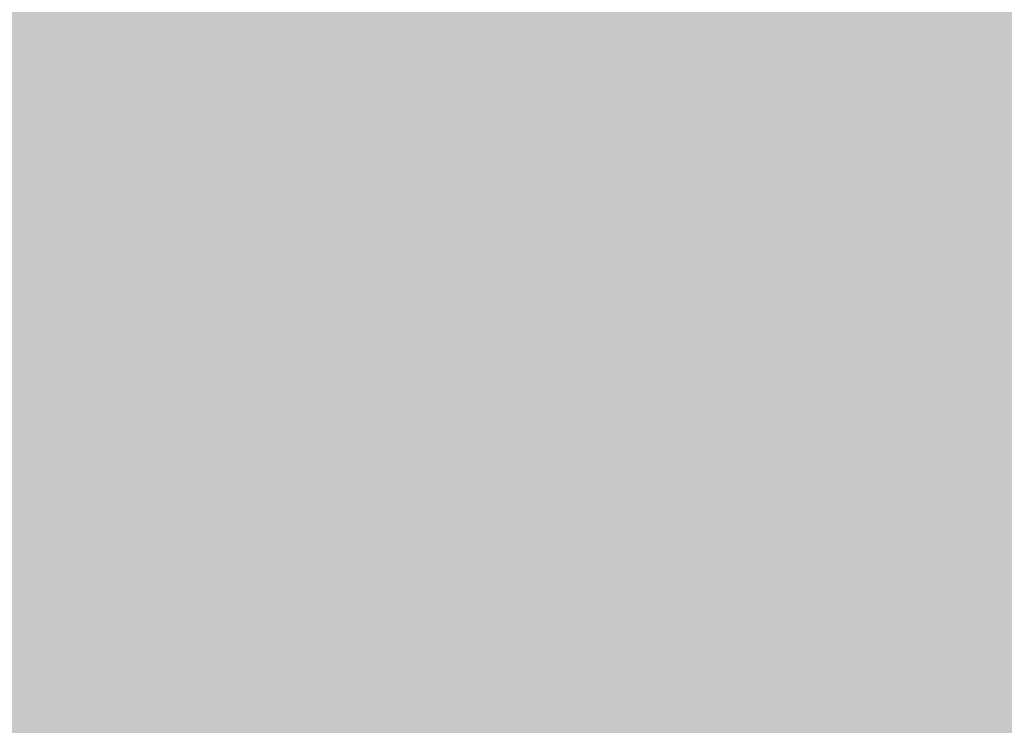
# Model space of a CAD drawing. Units: millimetres. Extents: x 0 to 2267, y 0 to 1823.
# Tile 77 of 256: x 1589.69 to 1600.37, y 1235.77 to 1243.41. Entities that reach past the tile are written whole.
import ezdxf

# ---------------------------------------------------------------- set-up
doc = ezdxf.new("R2010")
doc.units = ezdxf.units.MM
doc.header["$MEASUREMENT"] = 0
doc.layers.add('M-DIMS', color=2, linetype='Continuous', lineweight=25)
doc.layers.add('M-HATC', color=252, linetype='Continuous', lineweight=18)
doc.styles.get("Standard").update_dxf_attribs({"font": 'arial.ttf'})
doc.dimstyles.get("Standard").update_dxf_attribs({"dimtxt": 7, "dimasz": 4, "dimexe": 0.18, "dimexo": 0.0625, "dimgap": 0.09, "dimtad": 0, "dimdec": 0, "dimzin": 0, "dimdsep": 46, "dimtxsty": 'Standard', "dimcen": 0.09, "dimadec": 0, "dimazin": 0, "dimtfac": 1, "dimtdec": 0, "dimtofl": 0, "dimtmove": 0, "dimatfit": 3, "dimfxl": 1, "dimtolj": 1, "dimtzin": 0, "dimarcsym": 0})

# ---------------------------------------------------------------- blocks, each defined once
blk = doc.blocks.new('*D19')
at = {"layer": 'Defpoints', "color": 0, "transparency": 16777216}
for p in [(1605.34, 1483.304), (1445.529, 1333.885)]:
    blk.add_point(p, dxfattribs=at)
at = {"layer": 'M-DIMS', "color": 0, "lineweight": -2, "transparency": 16777216}
for p, q in [((1605.34, 1483.214), (1605.34, 1483.394)), ((1605.25, 1483.304), (1605.43, 1483.304)), ((1366.324, 1259.831), (1442.607, 1331.153))]:
    blk.add_line(p, q, dxfattribs=at)
at = {"layer": 'M-DIMS', "color": 0, "transparency": 16777216}
blk.add_solid([(1442.152, 1331.64), (1443.063, 1330.666), (1445.529, 1333.885)], dxfattribs=at)
at = {"layer": 'M-DIMS', "color": 0, "transparency": 16777216, "insert": (1349.643, 1244.233), "char_height": 7, "attachment_point": 5, "rotation": 43.0753}
blk.add_mtext('\\A1;2X R218.8', dxfattribs=at)

msp = doc.modelspace()

# ---------------------------------------------------------------- hatches: boundary and pattern name
at = {"layer": 'M-HATC'}
h = msp.add_hatch(color=256, dxfattribs=at)
h.dxf.hatch_style = 1
h.paths.add_polyline_path([(2065.771, 1618.062, 0.236068), (2055.771, 1638.062), (1381.087, 1638.062, 0.236068), (1371.087, 1618.062), (1371.087, 1603.062), (2055.771, 1603.062), (2065.771, 1603.062)])
h.paths.add_polyline_path([(2062.772, 1550.296), (2062.772, 1560.296), (1374.086, 1560.296), (1374.086, 1550.296), (1374.086, 1540.296), (1384.086, 1540.296), (1389.086, 1540.296), (2062.772, 1540.296)])
h.paths.add_polyline_path([(1930.929, 1282.766), (1505.929, 1282.766), (1587.628, 1235.597, 0.131652), (1600.128, 1232.247), (1836.73, 1232.247, 0.131652), (1849.23, 1235.597)])
h.paths.add_polyline_path([(1930.929, 1117.417), (1905.929, 1117.417), (1505.929, 1117.417), (1505.929, 1077.417), (1930.929, 1077.417)])
h = msp.add_hatch(color=256, dxfattribs=at)
h.dxf.hatch_style = 1
h.paths.add_polyline_path([(2055.771, 1603.062), (1381.087, 1603.062), (1381.087, 1598.062), (2055.771, 1598.062)])
h.paths.add_polyline_path([(2055.771, 1598.062), (1381.087, 1598.062), (1381.087, 1593.062), (2055.771, 1593.062)])
h.paths.add_polyline_path([(2051.307, 1536.761), (1385.55, 1536.761), (1385.55, 1526.761), (1387.55, 1526.761), (1388.537, 1525.053), (1385.332, 1521.233), (1385.332, 1521.223), (2050.254, 1522.749), (2048.321, 1525.053), (2049.307, 1526.761), (2051.307, 1526.761)])
edge = h.paths.add_edge_path()
edge.add_arc((1847.535, 1379.149), 135, 222.60306, 222.89085, ccw=False)
edge.add_line((1748.166, 1287.766), (1683.092, 1287.766))
edge.add_arc((1583.724, 1379.149), 135, 317.10915, 317.39694, ccw=False)
edge.add_arc((1678.969, 1290.671), 5, 222.8909, 317.1091, ccw=False)
edge.add_arc((1774.213, 1379.149), 135, 222.60306, 222.89085, ccw=False)
edge.add_line((1674.845, 1287.766), (1609.771, 1287.766))
edge.add_arc((1510.403, 1379.149), 135, 317.10915, 317.39694, ccw=False)
edge.add_arc((1605.647, 1290.671), 5, 222.8909, 317.1091, ccw=False)
edge.add_arc((1700.892, 1379.149), 135, 222.60306, 222.89085, ccw=False)
edge.add_line((1601.524, 1287.766), (1536.45, 1287.766))
edge.add_arc((1437.081, 1379.149), 135, 317.10915, 317.39694, ccw=False)
edge.add_arc((1532.326, 1290.671), 5, 222.8909, 317.1091, ccw=False)
edge.add_arc((1627.571, 1379.149), 135, 222.60306, 222.89085, ccw=False)
edge.add_line((1528.203, 1287.766), (1505.929, 1287.766))
edge.add_spline(control_points=[(1505.929, 1287.766), (1504.262, 1287.766), (1504.262, 1282.766), (1505.929, 1282.766)], knot_values=[0, 0, 0, 0, 5, 5, 5, 5], degree=3, periodic=0)
edge.add_line((1505.929, 1282.766), (1930.929, 1282.766))
edge.add_spline(control_points=[(1930.929, 1282.766), (1932.596, 1282.766), (1932.596, 1287.766), (1930.929, 1287.766)], knot_values=[0, 0, 0, 0, 5, 5, 5, 5], degree=3, periodic=0)
edge.add_line((1930.929, 1287.766), (1903.056, 1287.766))
edge.add_arc((1803.688, 1379.149), 135, 317.10915, 317.39694, ccw=False)
edge.add_arc((1898.932, 1290.671), 5, 222.8909, 317.1091, ccw=False)
edge.add_arc((1994.177, 1379.149), 135, 222.60306, 222.89085, ccw=False)
edge.add_line((1894.809, 1287.766), (1829.735, 1287.766))
edge.add_arc((1730.366, 1379.149), 135, 317.10915, 317.39694, ccw=False)
edge.add_arc((1825.611, 1290.671), 5, 222.8909, 317.1091, ccw=False)
edge.add_arc((1920.856, 1379.149), 135, 222.60306, 222.89085, ccw=False)
edge.add_line((1821.487, 1287.766), (1756.413, 1287.766))
edge.add_arc((1657.045, 1379.149), 135, 317.10915, 317.39694, ccw=False)
edge.add_arc((1752.29, 1290.671), 5, 222.8909, 317.1091, ccw=False)
edge = h.paths.add_edge_path()
edge.add_spline(control_points=[(1843.429, 1227.247), (1845.096, 1227.247), (1845.096, 1232.247), (1843.429, 1232.247)], knot_values=[0, 0, 0, 0, 5, 5, 5, 5], degree=3, periodic=0)
edge.add_line((1843.429, 1232.247), (1593.429, 1232.247))
edge.add_spline(control_points=[(1593.429, 1232.247), (1591.762, 1232.247), (1591.762, 1227.247), (1593.429, 1227.247)], knot_values=[0, 0, 0, 0, 5, 5, 5, 5], degree=3, periodic=0)
edge.add_line((1593.429, 1227.247), (1843.429, 1227.247))
h.paths.add_polyline_path([(1905.929, 1127.417), (1530.929, 1127.417, 0.414214), (1520.929, 1117.417), (1530.929, 1117.417), (1915.929, 1117.417, 0.414214)])
edge = h.paths.add_edge_path()
edge.add_arc((1397.086, 1498.408), 12.73, 90.7821, 190.8787, ccw=False)
edge.add_line((1396.912, 1511.136), (1428.01, 1511.349))
edge.add_line((1428.01, 1511.349), (1433.01, 1511.349))
edge.add_line((1433.01, 1511.349), (1434.439, 1511.349))
edge.add_arc((1419.474, 1498.08), 20, 41.561, 74.0821)
edge.add_line((1424.959, 1517.314), (1399.935, 1517.256))
edge.add_spline(control_points=[(1399.931, 1517.256), (1399.884, 1517.213), (1399.833, 1517.169), (1399.777, 1517.124)], knot_values=[11.567499, 11.567499, 11.567499, 11.567499, 11.814249, 11.814249, 11.814249, 11.814249], degree=3, periodic=0)
edge.add_spline(control_points=[(1399.633, 1517.01), (1399.583, 1516.972), (1399.531, 1516.934), (1399.476, 1516.895)], knot_values=[11.167718, 11.167718, 11.167718, 11.167718, 11.365188, 11.365188, 11.365188, 11.365188], degree=3, periodic=0)
edge.add_spline(control_points=[(1399.34, 1516.8), (1399.151, 1516.672), (1398.938, 1516.538), (1398.704, 1516.399)], knot_values=[10.376405, 10.376405, 10.376405, 10.376405, 11.00994, 11.00994, 11.00994, 11.00994], degree=3, periodic=0)
edge.add_spline(control_points=[(1398.657, 1516.372), (1398.579, 1516.326), (1398.498, 1516.28), (1398.415, 1516.233)], knot_values=[10.125175, 10.125175, 10.125175, 10.125175, 10.334406, 10.334406, 10.334406, 10.334406], degree=3, periodic=0)
edge.add_spline(control_points=[(1398.264, 1516.149), (1398.196, 1516.111), (1398.126, 1516.073), (1398.055, 1516.035)], knot_values=[9.832246, 9.832246, 9.832246, 9.832246, 9.999658, 9.999658, 9.999658, 9.999658], degree=3, periodic=0)
edge.add_spline(control_points=[(1397.999, 1516.005), (1397.731, 1515.862), (1397.446, 1515.717), (1397.147, 1515.571)], knot_values=[9.161808, 9.161808, 9.161808, 9.161808, 9.787769, 9.787769, 9.787769, 9.787769], degree=3, periodic=0)
edge.add_spline(control_points=[(1397.147, 1515.571), (1396.842, 1515.423), (1396.522, 1515.274), (1396.191, 1515.126)], knot_values=[8.524455, 8.524455, 8.524455, 8.524455, 9.161808, 9.161808, 9.161808, 9.161808], degree=3, periodic=0)
edge.add_spline(control_points=[(1396.078, 1515.076), (1395.985, 1515.035), (1395.892, 1514.994), (1395.798, 1514.953)], knot_values=[8.275193, 8.275193, 8.275193, 8.275193, 8.451726, 8.451726, 8.451726, 8.451726], degree=3, periodic=0)
edge.add_spline(control_points=[(1395.602, 1514.869), (1395.5, 1514.826), (1395.397, 1514.782), (1395.293, 1514.739)], knot_values=[7.962917, 7.962917, 7.962917, 7.962917, 8.152764, 8.152764, 8.152764, 8.152764], degree=3, periodic=0)
edge.add_spline(control_points=[(1395.212, 1514.706), (1394.828, 1514.547), (1394.435, 1514.393), (1394.036, 1514.244)], knot_values=[7.21254, 7.21254, 7.21254, 7.21254, 7.913148, 7.913148, 7.913148, 7.913148], degree=3, periodic=0)
edge.add_spline(control_points=[(1394.036, 1514.244), (1393.708, 1514.121), (1393.375, 1514.003), (1393.043, 1513.889)], knot_values=[6.633733, 6.633733, 6.633733, 6.633733, 7.21254, 7.21254, 7.21254, 7.21254], degree=3, periodic=0)
edge.add_spline(control_points=[(1392.821, 1513.815), (1392.72, 1513.781), (1392.618, 1513.748), (1392.517, 1513.715)], knot_values=[6.328796, 6.328796, 6.328796, 6.328796, 6.505493, 6.505493, 6.505493, 6.505493], degree=3, periodic=0)
edge.add_spline(control_points=[(1392.517, 1513.715), (1392.319, 1513.652), (1392.121, 1513.59), (1391.924, 1513.531)], knot_values=[5.984605, 5.984605, 5.984605, 5.984605, 6.328796, 6.328796, 6.328796, 6.328796], degree=3, periodic=0)
edge.add_spline(control_points=[(1391.792, 1513.491), (1391.312, 1513.35), (1390.838, 1513.224), (1390.378, 1513.117)], knot_values=[5.066697, 5.066697, 5.066697, 5.066697, 5.907055, 5.907055, 5.907055, 5.907055], degree=3, periodic=0)
edge.add_spline(control_points=[(1390.378, 1513.117), (1390.18, 1513.071), (1389.984, 1513.028), (1389.791, 1512.99)], knot_values=[4.70367, 4.70367, 4.70367, 4.70367, 5.066695, 5.066695, 5.066695, 5.066695], degree=3, periodic=0)
edge.add_spline(control_points=[(1389.422, 1512.92), (1389.246, 1512.889), (1389.073, 1512.862), (1388.904, 1512.838)], knot_values=[4.130571, 4.130571, 4.130571, 4.130571, 4.469816, 4.469816, 4.469816, 4.469816], degree=3, periodic=0)
edge.add_spline(control_points=[(1388.904, 1512.838), (1388.591, 1512.795), (1388.291, 1512.764), (1388.007, 1512.749)], knot_values=[3.504031, 3.504031, 3.504031, 3.504031, 4.130571, 4.130571, 4.130571, 4.130571], degree=3, periodic=0)
edge.add_spline(control_points=[(1387.936, 1512.746), (1387.854, 1512.742), (1387.773, 1512.74), (1387.694, 1512.739)], knot_values=[3.268866, 3.268866, 3.268866, 3.268866, 3.451164, 3.451164, 3.451164, 3.451164], degree=3, periodic=0)
edge.add_spline(control_points=[(1387.335, 1512.744), (1387.208, 1512.75), (1387.085, 1512.76), (1386.967, 1512.774)], knot_values=[2.670686, 2.670686, 2.670686, 2.670686, 2.984, 2.984, 2.984, 2.984], degree=3, periodic=0)
edge.add_spline(control_points=[(1386.833, 1512.792), (1386.821, 1512.794), (1386.809, 1512.796), (1386.797, 1512.798)], knot_values=[2.516981, 2.516981, 2.516981, 2.516981, 2.549528, 2.549528, 2.549528, 2.549528], degree=3, periodic=0)
edge.add_spline(control_points=[(1386.453, 1512.873), (1386.426, 1512.881), (1386.399, 1512.889), (1386.373, 1512.897)], knot_values=[2.095869, 2.095869, 2.095869, 2.095869, 2.17941, 2.17941, 2.17941, 2.17941], degree=3, periodic=0)
edge.add_spline(control_points=[(1386.069, 1513.019), (1386.063, 1513.022), (1386.058, 1513.025), (1386.052, 1513.028)], knot_values=[1.72453, 1.72453, 1.72453, 1.72453, 1.745933, 1.745933, 1.745933, 1.745933], degree=3, periodic=0)
edge.add_arc((1399.474, 1498.08), 20, 131.8243, 180)
edge.add_arc((1630.334, 1505.548), 250.971, 181.70518, 236.42798)
edge.add_arc((1605.34, 1483.304), 218.782, 238.66083, 243.34961)
edge.add_arc((1647.091, 1510.359), 262.899, 183.12984, 237.85344, ccw=False)
h.paths.add_polyline_path([(1406.537, 1391.964, 0.149382), (1491.551, 1296.442, -0.129517)], flags=17)
edge = h.paths.add_edge_path()
edge.add_arc((2037.384, 1498.08), 20, 0, 48.2659)
edge.add_spline(control_points=[(2050.697, 1513.005), (2050.651, 1512.985), (2050.603, 1512.966), (2050.554, 1512.948)], knot_values=[1.835652, 1.835652, 1.835652, 1.835652, 2.000781, 2.000781, 2.000781, 2.000781], degree=3, periodic=0)
edge.add_spline(control_points=[(2050.462, 1512.917), (2050.479, 1512.922), (2050.496, 1512.928), (2050.513, 1512.934)], knot_values=[2.045477, 2.045477, 2.045477, 2.045477, 2.101389, 2.101389, 2.101389, 2.101389], degree=3, periodic=0)
edge.add_spline(control_points=[(2050.129, 1512.834), (2050.198, 1512.847), (2050.266, 1512.862), (2050.331, 1512.879)], knot_values=[2.237629, 2.237629, 2.237629, 2.237629, 2.435841, 2.435841, 2.435841, 2.435841], degree=3, periodic=0)
edge.add_spline(control_points=[(2050.095, 1512.828), (2050.106, 1512.83), (2050.118, 1512.832), (2050.129, 1512.834)], knot_values=[2.435841, 2.435841, 2.435841, 2.435841, 2.468321, 2.468321, 2.468321, 2.468321], degree=3, periodic=0)
edge.add_spline(control_points=[(2049.784, 1512.785), (2049.855, 1512.792), (2049.924, 1512.801), (2049.992, 1512.811)], knot_values=[2.563852, 2.563852, 2.563852, 2.563852, 2.748541, 2.748541, 2.748541, 2.748541], degree=3, periodic=0)
edge.add_spline(control_points=[(2049.405, 1512.762), (2049.536, 1512.765), (2049.663, 1512.773), (2049.784, 1512.785)], knot_values=[2.748541, 2.748541, 2.748541, 2.748541, 3.064882, 3.064882, 3.064882, 3.064882], degree=3, periodic=0)
edge.add_spline(control_points=[(2049.17, 1512.76), (2049.234, 1512.759), (2049.297, 1512.759), (2049.358, 1512.761)], knot_values=[3.102309, 3.102309, 3.102309, 3.102309, 3.2503, 3.2503, 3.2503, 3.2503], degree=3, periodic=0)
edge.add_spline(control_points=[(2048.857, 1512.769), (2048.964, 1512.764), (2049.068, 1512.761), (2049.17, 1512.76)], knot_values=[3.2503, 3.2503, 3.2503, 3.2503, 3.486069, 3.486069, 3.486069, 3.486069], degree=3, periodic=0)
edge.add_spline(control_points=[(2048.692, 1512.779), (2048.373, 1512.801), (2048.035, 1512.841), (2047.682, 1512.897)], knot_values=[3.606429, 3.606429, 3.606429, 3.606429, 4.2989, 4.2989, 4.2989, 4.2989], degree=3, periodic=0)
edge.add_spline(control_points=[(2047.682, 1512.897), (2047.546, 1512.919), (2047.408, 1512.942), (2047.268, 1512.969)], knot_values=[4.2989, 4.2989, 4.2989, 4.2989, 4.565769, 4.565769, 4.565769, 4.565769], degree=3, periodic=0)
edge.add_spline(control_points=[(2047.268, 1512.969), (2047.145, 1512.991), (2047.021, 1513.016), (2046.895, 1513.042)], knot_values=[4.565769, 4.565769, 4.565769, 4.565769, 4.799971, 4.799971, 4.799971, 4.799971], degree=3, periodic=0)
edge.add_spline(control_points=[(2046.895, 1513.042), (2046.529, 1513.119), (2046.151, 1513.209), (2045.768, 1513.311)], knot_values=[4.799971, 4.799971, 4.799971, 4.799971, 5.483718, 5.483718, 5.483718, 5.483718], degree=3, periodic=0)
edge.add_spline(control_points=[(2045.768, 1513.311), (2045.372, 1513.415), (2044.97, 1513.532), (2044.566, 1513.659)], knot_values=[5.483718, 5.483718, 5.483718, 5.483718, 6.187866, 6.187866, 6.187866, 6.187866], degree=3, periodic=0)
edge.add_spline(control_points=[(2044.566, 1513.659), (2044.415, 1513.706), (2044.263, 1513.755), (2044.112, 1513.805)], knot_values=[6.187866, 6.187866, 6.187866, 6.187866, 6.451551, 6.451551, 6.451551, 6.451551], degree=3, periodic=0)
edge.add_spline(control_points=[(2044.112, 1513.805), (2043.997, 1513.843), (2043.882, 1513.881), (2043.767, 1513.92)], knot_values=[6.451551, 6.451551, 6.451551, 6.451551, 6.651434, 6.651434, 6.651434, 6.651434], degree=3, periodic=0)
edge.add_spline(control_points=[(2043.767, 1513.92), (2043.372, 1514.055), (2042.977, 1514.198), (2042.589, 1514.346)], knot_values=[6.651434, 6.651434, 6.651434, 6.651434, 7.338879, 7.338879, 7.338879, 7.338879], degree=3, periodic=0)
edge.add_spline(control_points=[(2042.589, 1514.346), (2042.164, 1514.507), (2041.746, 1514.675), (2041.341, 1514.846)], knot_values=[7.338879, 7.338879, 7.338879, 7.338879, 8.089209, 8.089209, 8.089209, 8.089209], degree=3, periodic=0)
edge.add_spline(control_points=[(2041.341, 1514.846), (2041.103, 1514.946), (2040.869, 1515.048), (2040.64, 1515.15)], knot_values=[8.089209, 8.089209, 8.089209, 8.089209, 8.529587, 8.529587, 8.529587, 8.529587], degree=3, periodic=0)
edge.add_spline(control_points=[(2040.51, 1515.209), (2040.082, 1515.402), (2039.675, 1515.597), (2039.295, 1515.789)], knot_values=[8.613818, 8.613818, 8.613818, 8.613818, 9.44571, 9.44571, 9.44571, 9.44571], degree=3, periodic=0)
edge.add_spline(control_points=[(2039.295, 1515.789), (2039.062, 1515.907), (2038.839, 1516.025), (2038.629, 1516.14)], knot_values=[9.44571, 9.44571, 9.44571, 9.44571, 9.956404, 9.956404, 9.956404, 9.956404], degree=3, periodic=0)
edge.add_spline(control_points=[(2038.629, 1516.14), (2038.519, 1516.2), (2038.412, 1516.26), (2038.309, 1516.319)], knot_values=[9.956404, 9.956404, 9.956404, 9.956404, 10.223542, 10.223542, 10.223542, 10.223542], degree=3, periodic=0)
edge.add_spline(control_points=[(2038.309, 1516.319), (2038.214, 1516.374), (2038.122, 1516.428), (2038.033, 1516.481)], knot_values=[10.223542, 10.223542, 10.223542, 10.223542, 10.47051, 10.47051, 10.47051, 10.47051], degree=3, periodic=0)
edge.add_spline(control_points=[(2038.033, 1516.481), (2037.786, 1516.63), (2037.564, 1516.773), (2037.372, 1516.909)], knot_values=[10.47051, 10.47051, 10.47051, 10.47051, 11.15767, 11.15767, 11.15767, 11.15767], degree=3, periodic=0)
edge.add_spline(control_points=[(2037.372, 1516.909), (2037.279, 1516.975), (2037.193, 1517.04), (2037.114, 1517.102)], knot_values=[11.15767, 11.15767, 11.15767, 11.15767, 11.49227, 11.49227, 11.49227, 11.49227], degree=3, periodic=0)
edge.add_spline(control_points=[(2036.856, 1517.326), (2036.915, 1517.269), (2036.981, 1517.21), (2037.056, 1517.149)], knot_values=[11.577341, 11.577341, 11.577341, 11.577341, 11.91035, 11.91035, 11.91035, 11.91035], degree=3, periodic=0)
edge.add_spline(control_points=[(2036.807, 1517.375), (2036.823, 1517.359), (2036.839, 1517.342), (2036.856, 1517.326)], knot_values=[11.91035, 11.91035, 11.91035, 11.91035, 12.007402, 12.007402, 12.007402, 12.007402], degree=3, periodic=0)
edge.add_spline(control_points=[(2036.702, 1517.494), (2036.71, 1517.483), (2036.72, 1517.472), (2036.729, 1517.461)], knot_values=[12.184155, 12.184155, 12.184155, 12.184155, 12.255409, 12.255409, 12.255409, 12.255409], degree=3, periodic=0)
edge.add_spline(control_points=[(2036.616, 1517.621), (2036.62, 1517.613), (2036.624, 1517.606), (2036.629, 1517.598)], knot_values=[12.487913, 12.487913, 12.487913, 12.487913, 12.541035, 12.541035, 12.541035, 12.541035], degree=3, periodic=0)
edge.add_spline(control_points=[(2036.563, 1517.786), (2036.564, 1517.779), (2036.564, 1517.773), (2036.565, 1517.766)], knot_values=[12.911761, 12.911761, 12.911761, 12.911761, 12.968286, 12.968286, 12.968286, 12.968286], degree=3, periodic=0)
edge.add_spline(control_points=[(2036.617, 1517.93), (2036.612, 1517.926), (2036.609, 1517.921), (2036.605, 1517.916)], knot_values=[13.382527, 13.382527, 13.382527, 13.382527, 13.433791, 13.433791, 13.433791, 13.433791], degree=3, periodic=0)
edge.add_spline(control_points=[(2036.749, 1518.017), (2036.736, 1518.012), (2036.724, 1518.006), (2036.712, 1518)], knot_values=[13.726299, 13.726299, 13.726299, 13.726299, 13.809928, 13.809928, 13.809928, 13.809928], degree=3, periodic=0)
edge.add_spline(control_points=[(2036.86, 1518.053), (2036.839, 1518.047), (2036.818, 1518.042), (2036.799, 1518.035)], knot_values=[13.910887, 13.910887, 13.910887, 13.910887, 14.02153, 14.02153, 14.02153, 14.02153], degree=3, periodic=0)
edge.add_line((2036.964, 1518.08), (2032.384, 1518.08))
edge.add_line((2032.384, 1518.08), (2027.384, 1518.08))
edge.add_line((2027.384, 1518.08), (2022.384, 1518.08))
edge.add_line((2022.384, 1518.08), (2017.384, 1518.08))
edge.add_arc((2017.384, 1498.08), 20, 90, 138.439)
edge.add_line((2002.419, 1511.349), (2003.848, 1511.349))
edge.add_line((2003.848, 1511.349), (2008.848, 1511.349))
edge.add_line((2008.848, 1511.349), (2039.772, 1511.138))
edge.add_arc((2039.772, 1498.408), 12.73, -10.8787, 90, ccw=False)
edge.add_arc((1789.767, 1510.359), 262.899, 302.14656, 356.87016, ccw=False)
edge.add_arc((1831.518, 1483.304), 218.782, 296.65039, 301.33917)
edge.add_arc((1806.524, 1505.548), 250.971, 303.57202, 358.29482)
h.paths.add_polyline_path([(2030.321, 1391.964, -0.129517), (1945.307, 1296.442, 0.149382)], flags=17)
edge = h.paths.add_edge_path()
edge.add_spline(control_points=[(2037.246, 1518.082), (2037.29, 1518.081), (2037.336, 1518.08), (2037.384, 1518.08)], knot_values=[0.000012, 0.000012, 0.000012, 0.000012, 0.144754, 0.144754, 0.144754, 0.144754], degree=3, periodic=0)
edge.add_line((2037.336, 1518.08), (2037.01, 1518.08))
edge.add_spline(control_points=[(2037.01, 1518.08), (2036.982, 1518.077), (2036.956, 1518.073), (2036.931, 1518.068)], knot_values=[14.13465, 14.13465, 14.13465, 14.13465, 14.247197, 14.247197, 14.247197, 14.247197], degree=3, periodic=0)
edge.add_spline(control_points=[(2036.931, 1518.068), (2036.928, 1518.067), (2036.924, 1518.067), (2036.921, 1518.066)], knot_values=[14.118315, 14.118315, 14.118315, 14.118315, 14.13465, 14.13465, 14.13465, 14.13465], degree=3, periodic=0)
edge.add_spline(control_points=[(2036.921, 1518.066), (2036.912, 1518.064), (2036.903, 1518.063), (2036.895, 1518.061)], knot_values=[14.078086, 14.078086, 14.078086, 14.078086, 14.118315, 14.118315, 14.118315, 14.118315], degree=3, periodic=0)
edge.add_spline(control_points=[(2036.895, 1518.061), (2036.883, 1518.058), (2036.872, 1518.056), (2036.86, 1518.053)], knot_values=[14.02153, 14.02153, 14.02153, 14.02153, 14.078086, 14.078086, 14.078086, 14.078086], degree=3, periodic=0)
edge.add_spline(control_points=[(2036.86, 1518.053), (2036.839, 1518.047), (2036.818, 1518.042), (2036.799, 1518.035)], knot_values=[13.910887, 13.910887, 13.910887, 13.910887, 14.02153, 14.02153, 14.02153, 14.02153], degree=3, periodic=0)
edge.add_spline(control_points=[(2036.799, 1518.035), (2036.798, 1518.035), (2036.797, 1518.035), (2036.797, 1518.035)], knot_values=[13.906906, 13.906906, 13.906906, 13.906906, 13.910887, 13.910887, 13.910887, 13.910887], degree=3, periodic=0)
edge.add_spline(control_points=[(2036.797, 1518.035), (2036.788, 1518.032), (2036.78, 1518.029), (2036.772, 1518.026)], knot_values=[13.857826, 13.857826, 13.857826, 13.857826, 13.906906, 13.906906, 13.906906, 13.906906], degree=3, periodic=0)
edge.add_spline(control_points=[(2036.772, 1518.026), (2036.764, 1518.023), (2036.756, 1518.02), (2036.749, 1518.017)], knot_values=[13.809928, 13.809928, 13.809928, 13.809928, 13.857826, 13.857826, 13.857826, 13.857826], degree=3, periodic=0)
edge.add_spline(control_points=[(2036.749, 1518.017), (2036.736, 1518.012), (2036.724, 1518.006), (2036.712, 1518)], knot_values=[13.726299, 13.726299, 13.726299, 13.726299, 13.809928, 13.809928, 13.809928, 13.809928], degree=3, periodic=0)
edge.add_spline(control_points=[(2036.712, 1518), (2036.712, 1518), (2036.712, 1518), (2036.711, 1518)], knot_values=[13.723993, 13.723993, 13.723993, 13.723993, 13.726299, 13.726299, 13.726299, 13.726299], degree=3, periodic=0)
edge.add_spline(control_points=[(2036.711, 1518), (2036.706, 1517.997), (2036.701, 1517.994), (2036.696, 1517.992)], knot_values=[13.686536, 13.686536, 13.686536, 13.686536, 13.723993, 13.723993, 13.723993, 13.723993], degree=3, periodic=0)
edge.add_spline(control_points=[(2036.696, 1517.992), (2036.692, 1517.989), (2036.687, 1517.987), (2036.683, 1517.984)], knot_values=[13.651251, 13.651251, 13.651251, 13.651251, 13.686536, 13.686536, 13.686536, 13.686536], degree=3, periodic=0)
edge.add_spline(control_points=[(2036.683, 1517.984), (2036.676, 1517.98), (2036.67, 1517.976), (2036.664, 1517.971)], knot_values=[13.596804, 13.596804, 13.596804, 13.596804, 13.651251, 13.651251, 13.651251, 13.651251], degree=3, periodic=0)
edge.add_spline(control_points=[(2036.664, 1517.971), (2036.664, 1517.971), (2036.663, 1517.971), (2036.663, 1517.971)], knot_values=[13.593956, 13.593956, 13.593956, 13.593956, 13.596804, 13.596804, 13.596804, 13.596804], degree=3, periodic=0)
edge.add_spline(control_points=[(2036.663, 1517.971), (2036.66, 1517.969), (2036.658, 1517.967), (2036.655, 1517.965)], knot_values=[13.570322, 13.570322, 13.570322, 13.570322, 13.593956, 13.593956, 13.593956, 13.593956], degree=3, periodic=0)
edge.add_spline(control_points=[(2036.655, 1517.965), (2036.653, 1517.963), (2036.65, 1517.961), (2036.647, 1517.959)], knot_values=[13.545477, 13.545477, 13.545477, 13.545477, 13.570322, 13.570322, 13.570322, 13.570322], degree=3, periodic=0)
edge.add_spline(control_points=[(2036.647, 1517.959), (2036.647, 1517.959), (2036.647, 1517.959), (2036.647, 1517.959)], knot_values=[13.543931, 13.543931, 13.543931, 13.543931, 13.545477, 13.545477, 13.545477, 13.545477], degree=3, periodic=0)
edge.add_spline(control_points=[(2036.647, 1517.959), (2036.641, 1517.954), (2036.636, 1517.949), (2036.631, 1517.945)], knot_values=[13.488237, 13.488237, 13.488237, 13.488237, 13.543931, 13.543931, 13.543931, 13.543931], degree=3, periodic=0)
edge.add_spline(control_points=[(2036.631, 1517.945), (2036.628, 1517.942), (2036.626, 1517.94), (2036.623, 1517.937)], knot_values=[13.460307, 13.460307, 13.460307, 13.460307, 13.488237, 13.488237, 13.488237, 13.488237], degree=3, periodic=0)
edge.add_spline(control_points=[(2036.623, 1517.937), (2036.622, 1517.936), (2036.62, 1517.934), (2036.618, 1517.932)], knot_values=[13.439712, 13.439712, 13.439712, 13.439712, 13.460307, 13.460307, 13.460307, 13.460307], degree=3, periodic=0)
edge.add_spline(control_points=[(2036.618, 1517.932), (2036.618, 1517.931), (2036.617, 1517.931), (2036.617, 1517.93)], knot_values=[13.433791, 13.433791, 13.433791, 13.433791, 13.439712, 13.439712, 13.439712, 13.439712], degree=3, periodic=0)
edge.add_spline(control_points=[(2036.617, 1517.93), (2036.612, 1517.926), (2036.609, 1517.921), (2036.605, 1517.916)], knot_values=[13.382527, 13.382527, 13.382527, 13.382527, 13.433791, 13.433791, 13.433791, 13.433791], degree=3, periodic=0)
edge.add_spline(control_points=[(2036.605, 1517.916), (2036.603, 1517.913), (2036.6, 1517.91), (2036.598, 1517.907)], knot_values=[13.350017, 13.350017, 13.350017, 13.350017, 13.382527, 13.382527, 13.382527, 13.382527], degree=3, periodic=0)
edge.add_spline(control_points=[(2036.598, 1517.907), (2036.597, 1517.906), (2036.596, 1517.904), (2036.595, 1517.903)], knot_values=[13.333922, 13.333922, 13.333922, 13.333922, 13.350017, 13.350017, 13.350017, 13.350017], degree=3, periodic=0)
edge.add_spline(control_points=[(2036.595, 1517.903), (2036.595, 1517.902), (2036.594, 1517.901), (2036.593, 1517.9)], knot_values=[13.323828, 13.323828, 13.323828, 13.323828, 13.333922, 13.333922, 13.333922, 13.333922], degree=3, periodic=0)
edge.add_spline(control_points=[(2036.593, 1517.9), (2036.59, 1517.895), (2036.588, 1517.891), (2036.585, 1517.886)], knot_values=[13.277545, 13.277545, 13.277545, 13.277545, 13.323828, 13.323828, 13.323828, 13.323828], degree=3, periodic=0)
edge.add_spline(control_points=[(2036.585, 1517.886), (2036.584, 1517.883), (2036.582, 1517.879), (2036.58, 1517.875)], knot_values=[13.240119, 13.240119, 13.240119, 13.240119, 13.277545, 13.277545, 13.277545, 13.277545], degree=3, periodic=0)
edge.add_spline(control_points=[(2036.58, 1517.875), (2036.58, 1517.874), (2036.579, 1517.873), (2036.578, 1517.872)], knot_values=[13.228211, 13.228211, 13.228211, 13.228211, 13.240119, 13.240119, 13.240119, 13.240119], degree=3, periodic=0)
edge.add_spline(control_points=[(2036.578, 1517.872), (2036.578, 1517.87), (2036.577, 1517.869), (2036.577, 1517.868)], knot_values=[13.215717, 13.215717, 13.215717, 13.215717, 13.228211, 13.228211, 13.228211, 13.228211], degree=3, periodic=0)
edge.add_spline(control_points=[(2036.577, 1517.868), (2036.575, 1517.864), (2036.574, 1517.86), (2036.573, 1517.857)], knot_values=[13.179847, 13.179847, 13.179847, 13.179847, 13.215717, 13.215717, 13.215717, 13.215717], degree=3, periodic=0)
edge.add_spline(control_points=[(2036.573, 1517.857), (2036.571, 1517.851), (2036.57, 1517.846), (2036.569, 1517.841)], knot_values=[13.132017, 13.132017, 13.132017, 13.132017, 13.179847, 13.179847, 13.179847, 13.179847], degree=3, periodic=0)
edge.add_spline(control_points=[(2036.569, 1517.841), (2036.568, 1517.84), (2036.568, 1517.839), (2036.568, 1517.838)], knot_values=[13.122482, 13.122482, 13.122482, 13.122482, 13.132017, 13.132017, 13.132017, 13.132017], degree=3, periodic=0)
edge.add_spline(control_points=[(2036.568, 1517.838), (2036.568, 1517.836), (2036.567, 1517.835), (2036.567, 1517.833)], knot_values=[13.105592, 13.105592, 13.105592, 13.105592, 13.122482, 13.122482, 13.122482, 13.122482], degree=3, periodic=0)
edge.add_spline(control_points=[(2036.567, 1517.833), (2036.566, 1517.829), (2036.566, 1517.826), (2036.565, 1517.822)], knot_values=[13.074063, 13.074063, 13.074063, 13.074063, 13.105592, 13.105592, 13.105592, 13.105592], degree=3, periodic=0)
edge.add_spline(control_points=[(2036.565, 1517.822), (2036.565, 1517.822), (2036.565, 1517.822), (2036.565, 1517.822)], knot_values=[13.074043, 13.074043, 13.074043, 13.074043, 13.074063, 13.074063, 13.074063, 13.074063], degree=3, periodic=0)
edge.add_spline(control_points=[(2036.565, 1517.822), (2036.564, 1517.816), (2036.564, 1517.811), (2036.564, 1517.805)], knot_values=[13.021884, 13.021884, 13.021884, 13.021884, 13.074043, 13.074043, 13.074043, 13.074043], degree=3, periodic=0)
edge.add_spline(control_points=[(2036.564, 1517.805), (2036.564, 1517.804), (2036.564, 1517.803), (2036.564, 1517.803)], knot_values=[13.01674, 13.01674, 13.01674, 13.01674, 13.021884, 13.021884, 13.021884, 13.021884], degree=3, periodic=0)
edge.add_spline(control_points=[(2036.564, 1517.803), (2036.563, 1517.801), (2036.563, 1517.798), (2036.563, 1517.796)], knot_values=[12.996438, 12.996438, 12.996438, 12.996438, 13.01674, 13.01674, 13.01674, 13.01674], degree=3, periodic=0)
edge.add_spline(control_points=[(2036.563, 1517.796), (2036.563, 1517.793), (2036.563, 1517.789), (2036.563, 1517.786)], knot_values=[12.968286, 12.968286, 12.968286, 12.968286, 12.996438, 12.996438, 12.996438, 12.996438], degree=3, periodic=0)
edge.add_spline(control_points=[(2036.563, 1517.786), (2036.564, 1517.779), (2036.564, 1517.773), (2036.565, 1517.766)], knot_values=[12.911761, 12.911761, 12.911761, 12.911761, 12.968286, 12.968286, 12.968286, 12.968286], degree=3, periodic=0)
edge.add_spline(control_points=[(2036.565, 1517.766), (2036.565, 1517.766), (2036.565, 1517.766), (2036.565, 1517.766)], knot_values=[12.911017, 12.911017, 12.911017, 12.911017, 12.911761, 12.911761, 12.911761, 12.911761], degree=3, periodic=0)
edge.add_spline(control_points=[(2036.565, 1517.766), (2036.565, 1517.762), (2036.566, 1517.759), (2036.566, 1517.756)], knot_values=[12.88528, 12.88528, 12.88528, 12.88528, 12.911017, 12.911017, 12.911017, 12.911017], degree=3, periodic=0)
edge.add_spline(control_points=[(2036.566, 1517.756), (2036.567, 1517.753), (2036.567, 1517.751), (2036.568, 1517.748)], knot_values=[12.862519, 12.862519, 12.862519, 12.862519, 12.88528, 12.88528, 12.88528, 12.88528], degree=3, periodic=0)
edge.add_spline(control_points=[(2036.568, 1517.748), (2036.568, 1517.747), (2036.568, 1517.747), (2036.568, 1517.746)], knot_values=[12.858885, 12.858885, 12.858885, 12.858885, 12.862519, 12.862519, 12.862519, 12.862519], degree=3, periodic=0)
edge.add_spline(control_points=[(2036.568, 1517.746), (2036.569, 1517.74), (2036.571, 1517.733), (2036.572, 1517.726)], knot_values=[12.8053, 12.8053, 12.8053, 12.8053, 12.858885, 12.858885, 12.858885, 12.858885], degree=3, periodic=0)
edge.add_spline(control_points=[(2036.572, 1517.726), (2036.573, 1517.723), (2036.574, 1517.719), (2036.576, 1517.715)], knot_values=[12.775176, 12.775176, 12.775176, 12.775176, 12.8053, 12.8053, 12.8053, 12.8053], degree=3, periodic=0)
edge.add_spline(control_points=[(2036.576, 1517.715), (2036.576, 1517.713), (2036.577, 1517.71), (2036.578, 1517.708)], knot_values=[12.756759, 12.756759, 12.756759, 12.756759, 12.775176, 12.775176, 12.775176, 12.775176], degree=3, periodic=0)
edge.add_spline(control_points=[(2036.578, 1517.708), (2036.578, 1517.707), (2036.578, 1517.706), (2036.579, 1517.705)], knot_values=[12.748742, 12.748742, 12.748742, 12.748742, 12.756759, 12.756759, 12.756759, 12.756759], degree=3, periodic=0)
edge.add_spline(control_points=[(2036.579, 1517.705), (2036.581, 1517.698), (2036.583, 1517.692), (2036.586, 1517.685)], knot_values=[12.69959, 12.69959, 12.69959, 12.69959, 12.748742, 12.748742, 12.748742, 12.748742], degree=3, periodic=0)
edge.add_spline(control_points=[(2036.586, 1517.685), (2036.588, 1517.68), (2036.59, 1517.675), (2036.592, 1517.669)], knot_values=[12.659038, 12.659038, 12.659038, 12.659038, 12.69959, 12.69959, 12.69959, 12.69959], degree=3, periodic=0)
edge.add_spline(control_points=[(2036.592, 1517.669), (2036.594, 1517.665), (2036.596, 1517.66), (2036.598, 1517.656)], knot_values=[12.626806, 12.626806, 12.626806, 12.626806, 12.659038, 12.659038, 12.659038, 12.659038], degree=3, periodic=0)
edge.add_spline(control_points=[(2036.598, 1517.656), (2036.598, 1517.655), (2036.599, 1517.654), (2036.599, 1517.653)], knot_values=[12.619394, 12.619394, 12.619394, 12.619394, 12.626806, 12.626806, 12.626806, 12.626806], degree=3, periodic=0)
edge.add_spline(control_points=[(2036.599, 1517.653), (2036.604, 1517.642), (2036.61, 1517.632), (2036.616, 1517.621)], knot_values=[12.541039, 12.541039, 12.541039, 12.541039, 12.619394, 12.619394, 12.619394, 12.619394], degree=3, periodic=0)
edge.add_spline(control_points=[(2036.616, 1517.621), (2036.616, 1517.621), (2036.616, 1517.621), (2036.616, 1517.621)], knot_values=[12.541035, 12.541035, 12.541035, 12.541035, 12.541039, 12.541039, 12.541039, 12.541039], degree=3, periodic=0)
edge.add_spline(control_points=[(2036.616, 1517.621), (2036.62, 1517.613), (2036.624, 1517.606), (2036.629, 1517.598)], knot_values=[12.487913, 12.487913, 12.487913, 12.487913, 12.541035, 12.541035, 12.541035, 12.541035], degree=3, periodic=0)
edge.add_spline(control_points=[(2036.629, 1517.598), (2036.633, 1517.592), (2036.637, 1517.585), (2036.641, 1517.579)], knot_values=[12.443982, 12.443982, 12.443982, 12.443982, 12.487913, 12.487913, 12.487913, 12.487913], degree=3, periodic=0)
edge.add_spline(control_points=[(2036.641, 1517.579), (2036.641, 1517.578), (2036.642, 1517.576), (2036.643, 1517.575)], knot_values=[12.434996, 12.434996, 12.434996, 12.434996, 12.443982, 12.443982, 12.443982, 12.443982], degree=3, periodic=0)
edge.add_spline(control_points=[(2036.643, 1517.575), (2036.653, 1517.56), (2036.664, 1517.544), (2036.676, 1517.528)], knot_values=[12.329647, 12.329647, 12.329647, 12.329647, 12.434996, 12.434996, 12.434996, 12.434996], degree=3, periodic=0)
edge.add_spline(control_points=[(2036.676, 1517.528), (2036.684, 1517.517), (2036.693, 1517.505), (2036.702, 1517.494)], knot_values=[12.255409, 12.255409, 12.255409, 12.255409, 12.329647, 12.329647, 12.329647, 12.329647], degree=3, periodic=0)
edge.add_spline(control_points=[(2036.702, 1517.494), (2036.71, 1517.483), (2036.72, 1517.472), (2036.729, 1517.461)], knot_values=[12.184155, 12.184155, 12.184155, 12.184155, 12.255409, 12.255409, 12.255409, 12.255409], degree=3, periodic=0)
edge.add_spline(control_points=[(2036.729, 1517.461), (2036.744, 1517.444), (2036.759, 1517.426), (2036.775, 1517.409)], knot_values=[12.075961, 12.075961, 12.075961, 12.075961, 12.184155, 12.184155, 12.184155, 12.184155], degree=3, periodic=0)
edge.add_spline(control_points=[(2036.775, 1517.409), (2036.776, 1517.407), (2036.777, 1517.406), (2036.778, 1517.405)], knot_values=[12.069502, 12.069502, 12.069502, 12.069502, 12.075961, 12.075961, 12.075961, 12.075961], degree=3, periodic=0)
edge.add_spline(control_points=[(2036.778, 1517.405), (2036.788, 1517.395), (2036.797, 1517.385), (2036.807, 1517.375)], knot_values=[12.007402, 12.007402, 12.007402, 12.007402, 12.069502, 12.069502, 12.069502, 12.069502], degree=3, periodic=0)
edge.add_spline(control_points=[(2036.807, 1517.375), (2036.823, 1517.359), (2036.839, 1517.342), (2036.856, 1517.326)], knot_values=[11.91035, 11.91035, 11.91035, 11.91035, 12.007402, 12.007402, 12.007402, 12.007402], degree=3, periodic=0)
edge.add_spline(control_points=[(2036.856, 1517.326), (2036.915, 1517.269), (2036.981, 1517.21), (2037.056, 1517.149)], knot_values=[11.577341, 11.577341, 11.577341, 11.577341, 11.91035, 11.91035, 11.91035, 11.91035], degree=3, periodic=0)
edge.add_spline(control_points=[(2037.056, 1517.149), (2037.075, 1517.134), (2037.094, 1517.118), (2037.114, 1517.102)], knot_values=[11.49227, 11.49227, 11.49227, 11.49227, 11.577341, 11.577341, 11.577341, 11.577341], degree=3, periodic=0)
edge.add_spline(control_points=[(2037.114, 1517.102), (2037.193, 1517.04), (2037.279, 1516.975), (2037.372, 1516.909)], knot_values=[11.15767, 11.15767, 11.15767, 11.15767, 11.49227, 11.49227, 11.49227, 11.49227], degree=3, periodic=0)
edge.add_spline(control_points=[(2037.372, 1516.909), (2037.564, 1516.773), (2037.786, 1516.63), (2038.033, 1516.481)], knot_values=[10.47051, 10.47051, 10.47051, 10.47051, 11.15767, 11.15767, 11.15767, 11.15767], degree=3, periodic=0)
edge.add_spline(control_points=[(2038.033, 1516.481), (2038.122, 1516.428), (2038.214, 1516.374), (2038.309, 1516.319)], knot_values=[10.223542, 10.223542, 10.223542, 10.223542, 10.47051, 10.47051, 10.47051, 10.47051], degree=3, periodic=0)
edge.add_spline(control_points=[(2038.309, 1516.319), (2038.412, 1516.26), (2038.519, 1516.2), (2038.629, 1516.14)], knot_values=[9.956404, 9.956404, 9.956404, 9.956404, 10.223542, 10.223542, 10.223542, 10.223542], degree=3, periodic=0)
edge.add_spline(control_points=[(2038.629, 1516.14), (2038.839, 1516.025), (2039.062, 1515.907), (2039.295, 1515.789)], knot_values=[9.44571, 9.44571, 9.44571, 9.44571, 9.956404, 9.956404, 9.956404, 9.956404], degree=3, periodic=0)
edge.add_spline(control_points=[(2039.295, 1515.789), (2039.675, 1515.597), (2040.082, 1515.402), (2040.51, 1515.209)], knot_values=[8.613818, 8.613818, 8.613818, 8.613818, 9.44571, 9.44571, 9.44571, 9.44571], degree=3, periodic=0)
edge.add_spline(control_points=[(2040.51, 1515.209), (2040.553, 1515.189), (2040.597, 1515.17), (2040.64, 1515.15)], knot_values=[8.529587, 8.529587, 8.529587, 8.529587, 8.613818, 8.613818, 8.613818, 8.613818], degree=3, periodic=0)
edge.add_spline(control_points=[(2040.64, 1515.15), (2040.869, 1515.048), (2041.103, 1514.946), (2041.341, 1514.846)], knot_values=[8.089209, 8.089209, 8.089209, 8.089209, 8.529587, 8.529587, 8.529587, 8.529587], degree=3, periodic=0)
edge.add_spline(control_points=[(2041.341, 1514.846), (2041.746, 1514.675), (2042.164, 1514.507), (2042.589, 1514.346)], knot_values=[7.338879, 7.338879, 7.338879, 7.338879, 8.089209, 8.089209, 8.089209, 8.089209], degree=3, periodic=0)
edge.add_spline(control_points=[(2042.589, 1514.346), (2042.977, 1514.198), (2043.372, 1514.055), (2043.767, 1513.92)], knot_values=[6.651434, 6.651434, 6.651434, 6.651434, 7.338879, 7.338879, 7.338879, 7.338879], degree=3, periodic=0)
edge.add_spline(control_points=[(2043.767, 1513.92), (2043.882, 1513.881), (2043.997, 1513.843), (2044.112, 1513.805)], knot_values=[6.451551, 6.451551, 6.451551, 6.451551, 6.651434, 6.651434, 6.651434, 6.651434], degree=3, periodic=0)
edge.add_spline(control_points=[(2044.112, 1513.805), (2044.263, 1513.755), (2044.415, 1513.706), (2044.566, 1513.659)], knot_values=[6.187866, 6.187866, 6.187866, 6.187866, 6.451551, 6.451551, 6.451551, 6.451551], degree=3, periodic=0)
edge.add_spline(control_points=[(2044.566, 1513.659), (2044.97, 1513.532), (2045.372, 1513.415), (2045.768, 1513.311)], knot_values=[5.483718, 5.483718, 5.483718, 5.483718, 6.187866, 6.187866, 6.187866, 6.187866], degree=3, periodic=0)
edge.add_spline(control_points=[(2045.768, 1513.311), (2046.151, 1513.209), (2046.529, 1513.119), (2046.895, 1513.042)], knot_values=[4.799971, 4.799971, 4.799971, 4.799971, 5.483718, 5.483718, 5.483718, 5.483718], degree=3, periodic=0)
edge.add_spline(control_points=[(2046.895, 1513.042), (2047.021, 1513.016), (2047.145, 1512.991), (2047.268, 1512.969)], knot_values=[4.565769, 4.565769, 4.565769, 4.565769, 4.799971, 4.799971, 4.799971, 4.799971], degree=3, periodic=0)
edge.add_spline(control_points=[(2047.268, 1512.969), (2047.408, 1512.942), (2047.546, 1512.919), (2047.682, 1512.897)], knot_values=[4.2989, 4.2989, 4.2989, 4.2989, 4.565769, 4.565769, 4.565769, 4.565769], degree=3, periodic=0)
edge.add_spline(control_points=[(2047.682, 1512.897), (2048.035, 1512.841), (2048.373, 1512.801), (2048.692, 1512.779)], knot_values=[3.606429, 3.606429, 3.606429, 3.606429, 4.2989, 4.2989, 4.2989, 4.2989], degree=3, periodic=0)
edge.add_spline(control_points=[(2048.692, 1512.779), (2048.748, 1512.775), (2048.803, 1512.772), (2048.857, 1512.769)], knot_values=[3.486069, 3.486069, 3.486069, 3.486069, 3.606429, 3.606429, 3.606429, 3.606429], degree=3, periodic=0)
edge.add_spline(control_points=[(2048.857, 1512.769), (2048.964, 1512.764), (2049.068, 1512.761), (2049.17, 1512.76)], knot_values=[3.2503, 3.2503, 3.2503, 3.2503, 3.486069, 3.486069, 3.486069, 3.486069], degree=3, periodic=0)
edge.add_spline(control_points=[(2049.17, 1512.76), (2049.234, 1512.759), (2049.297, 1512.759), (2049.358, 1512.761)], knot_values=[3.102309, 3.102309, 3.102309, 3.102309, 3.2503, 3.2503, 3.2503, 3.2503], degree=3, periodic=0)
edge.add_spline(control_points=[(2049.358, 1512.761), (2049.374, 1512.761), (2049.39, 1512.761), (2049.405, 1512.762)], knot_values=[3.064882, 3.064882, 3.064882, 3.064882, 3.102309, 3.102309, 3.102309, 3.102309], degree=3, periodic=0)
edge.add_spline(control_points=[(2049.405, 1512.762), (2049.536, 1512.765), (2049.663, 1512.773), (2049.784, 1512.785)], knot_values=[2.748541, 2.748541, 2.748541, 2.748541, 3.064882, 3.064882, 3.064882, 3.064882], degree=3, periodic=0)
edge.add_spline(control_points=[(2049.784, 1512.785), (2049.855, 1512.792), (2049.924, 1512.801), (2049.992, 1512.811)], knot_values=[2.563852, 2.563852, 2.563852, 2.563852, 2.748541, 2.748541, 2.748541, 2.748541], degree=3, periodic=0)
edge.add_spline(control_points=[(2049.992, 1512.811), (2050.026, 1512.816), (2050.061, 1512.822), (2050.095, 1512.828)], knot_values=[2.468321, 2.468321, 2.468321, 2.468321, 2.563852, 2.563852, 2.563852, 2.563852], degree=3, periodic=0)
edge.add_spline(control_points=[(2050.095, 1512.828), (2050.106, 1512.83), (2050.118, 1512.832), (2050.129, 1512.834)], knot_values=[2.435841, 2.435841, 2.435841, 2.435841, 2.468321, 2.468321, 2.468321, 2.468321], degree=3, periodic=0)
edge.add_spline(control_points=[(2050.129, 1512.834), (2050.198, 1512.847), (2050.266, 1512.862), (2050.331, 1512.879)], knot_values=[2.237629, 2.237629, 2.237629, 2.237629, 2.435841, 2.435841, 2.435841, 2.435841], degree=3, periodic=0)
edge.add_spline(control_points=[(2050.331, 1512.879), (2050.375, 1512.891), (2050.419, 1512.903), (2050.462, 1512.917)], knot_values=[2.101389, 2.101389, 2.101389, 2.101389, 2.237629, 2.237629, 2.237629, 2.237629], degree=3, periodic=0)
edge.add_spline(control_points=[(2050.462, 1512.917), (2050.479, 1512.922), (2050.496, 1512.928), (2050.513, 1512.934)], knot_values=[2.045477, 2.045477, 2.045477, 2.045477, 2.101389, 2.101389, 2.101389, 2.101389], degree=3, periodic=0)
edge.add_spline(control_points=[(2050.513, 1512.934), (2050.527, 1512.938), (2050.54, 1512.943), (2050.554, 1512.948)], knot_values=[2.000781, 2.000781, 2.000781, 2.000781, 2.045477, 2.045477, 2.045477, 2.045477], degree=3, periodic=0)
edge.add_spline(control_points=[(2050.554, 1512.948), (2050.603, 1512.966), (2050.651, 1512.985), (2050.697, 1513.005)], knot_values=[1.835652, 1.835652, 1.835652, 1.835652, 2.000781, 2.000781, 2.000781, 2.000781], degree=3, periodic=0)
edge.add_arc((2037.384, 1498.08), 20, 48.2659, 90.1299)
edge = h.paths.add_edge_path(flags=16)
edge.add_spline(control_points=[(1386.139, 1512.986), (1388.92, 1511.739), (1398.039, 1515.519), (1399.931, 1517.256)], knot_values=[1.831046, 1.831046, 1.831046, 1.831046, 11.814249, 11.814249, 11.814249, 11.814249], degree=3, periodic=0)
edge.add_line((1399.931, 1517.256), (1393.743, 1517.242))
edge.add_arc((1399.474, 1498.08), 20, 106.6501, 131.8173)

# ---------------------------------------------------------------- dimensions: what is measured, and where the dimension line sits
at = {"layer": 'M-DIMS'}
dim = msp.add_radius_dim(center=(1605.34, 1483.304), mpoint=(1445.529, 1333.885), text='2X <>', dimstyle='Standard', override={"dimdec": 1, "dimlfac": 1, "dimrnd": 0, "dimzin": 0, "dimdsep": 46, "dimlunit": 2}, dxfattribs=at)
dim.commit()
dim.dimension.update_dxf_attribs({"geometry": '*D19', "text_midpoint": (1349.643, 1244.233), "dimtype": 164})

doc.saveas('drawing.dxf')
